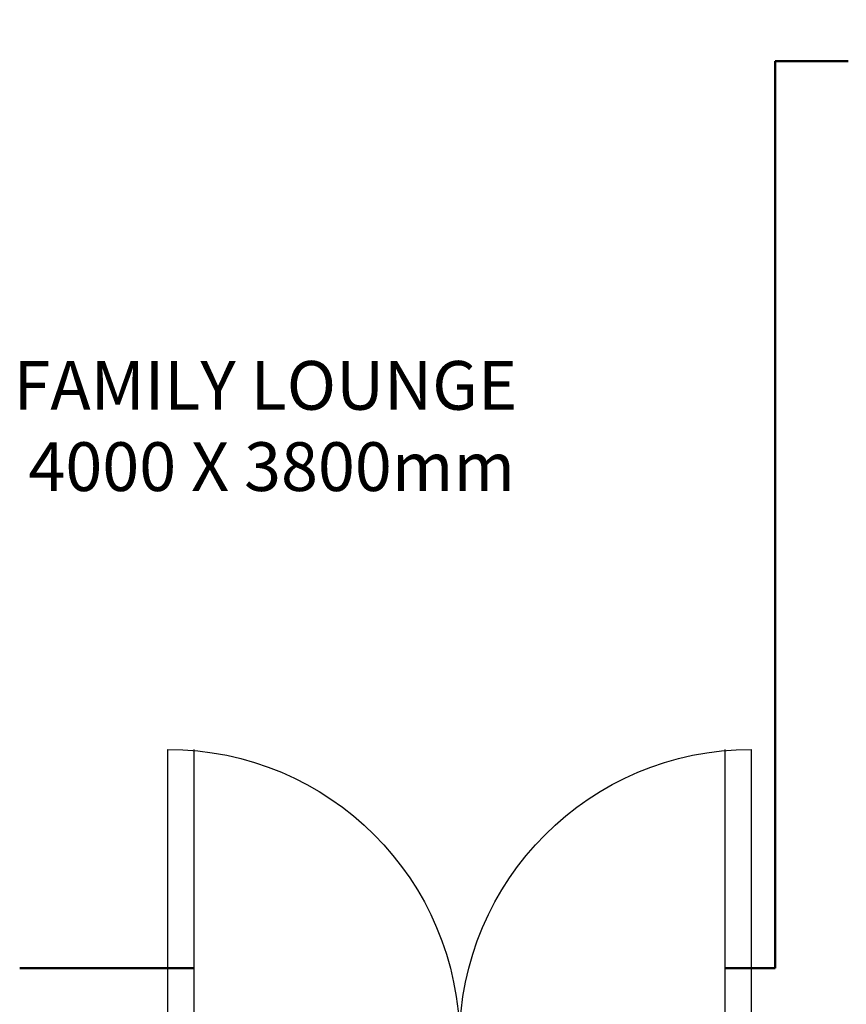
# Model space of a CAD drawing. Units: millimetres. Extents: x -857 to 54106, y -13666 to 13947.
# Tile 10 of 41: x 9086 to 11637, y 5442 to 8482. Entities that reach past the tile are written whole.
import ezdxf

# ---------------------------------------------------------------- set-up
doc = ezdxf.new("R2010")
doc.units = ezdxf.units.MM
for name, color, linetype, lineweight in [('A-AREA-IDEN', 3, 'Continuous', 18), ('A-DOOR', 1, 'Continuous', 25), ('A-FLOR-PATT', 252, 'Continuous', 13), ('A-WALL', 7, 'Continuous', 50)]:
    doc.layers.add(name, color=color, linetype=linetype, lineweight=lineweight)
doc.styles.get("Standard").update_dxf_attribs({"font": 'arial.ttf'})

msp = doc.modelspace()

# ---------------------------------------------------------------- hatches: boundary and pattern name
at = {"layer": 'A-FLOR-PATT'}
h = msp.add_hatch(dxfattribs=at)
h.set_pattern_fill('CROSS', color=256, scale=50)
h.set_pattern_definition([(0, (-5489.92, -2561.3), (317.5, 317.5), [158.75, -476.25]), (90, (-5410.54, -2640.7), (-317.5, 317.5), [158.75, -476.25])])
h.paths.add_polyline_path([(16392.264, 9351.555), (14441.85, 9351.555), (13967.28, 9353.369), (13967.28, 9241.901), (13967.28, 8421.901), (13967.28, 6326.555), (16392.264, 6326.555)])
h.paths.add_polyline_path([(16392.264, 12804.231), (14667.264, 12804.231), (14667.264, 12374.147, -0.32131534), (15142.28, 11711.288), (14667.264, 11711.288), (14667.264, 11601.555), (16392.264, 11601.555)])
h.paths.add_polyline_path([(11417.28, 12804.231), (8617.28, 12804.231), (8617.28, 11804.231), (9371.341, 11804.231), (9371.341, 11750.152), (10571.341, 11750.152), (10571.341, 11804.231), (11417.28, 11804.231)])

# ---------------------------------------------------------------- linework, layer by layer
at = {"layer": 'A-DOOR'}
msp.add_lwpolyline([(9623.585, 6229.231), (9623.585, 5329.231), (9543.585, 5329.231), (9543.585, 6229.231, -0.41421356), (10443.585, 5329.231, -0.41421356), (11343.585, 6229.231), (11343.585, 5329.231), (11263.585, 5329.231), (11263.585, 6229.231)], format="xyb", dxfattribs=at)
at = {"layer": 'A-WALL'}
for p, q in [((11417.28, 5554.231), (11417.28, 8354.231)), ((11642.28, 8354.231), (11417.28, 8354.231)), ((9086.254, 5554.231), (9623.585, 5554.231)), ((9623.585, 5554.231), (9469.891, 5554.231)), ((11343.585, 5554.231), (11263.585, 5554.231)), ((11417.28, 5554.231), (11343.585, 5554.231))]:
    msp.add_line(p, q, dxfattribs=at)

# ---------------------------------------------------------------- texts
at = {"layer": 'A-AREA-IDEN', "insert": (9067.268, 7428.283), "char_height": 150.48461, "attachment_point": 1}
msp.add_mtext_dynamic_manual_height_columns('\\pxt0;FAMILY LOUNGE\\P 4000 X 3800mm', width=2554.22693, gutter_width=18810.576, heights=[2595.835], dxfattribs=at)

doc.saveas('drawing.dxf')
